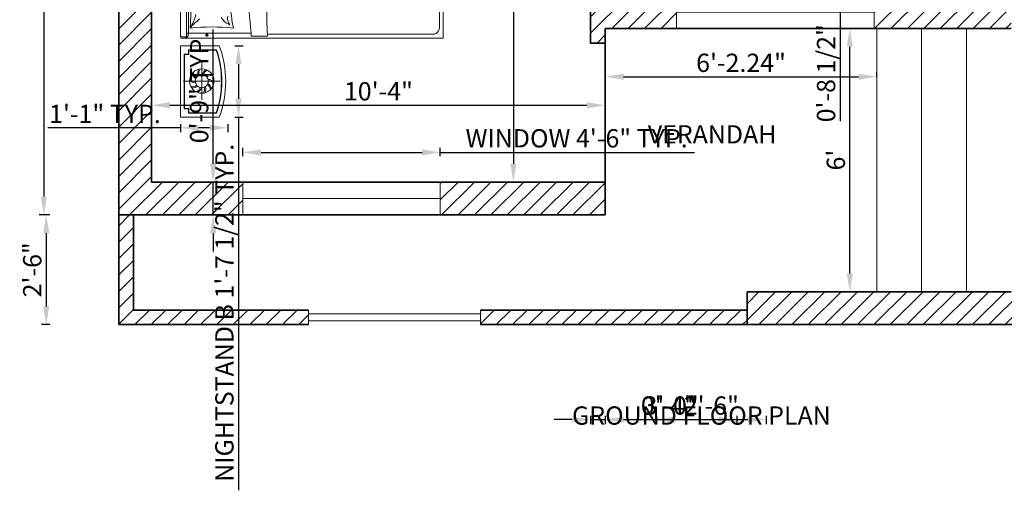
# Model space of a CAD drawing. Units: inches. Extents: x -196 to 219, y -474 to 80.
# Tile 1 of 4: x -196 to 73, y -474 to -346. Entities that reach past the tile are written whole.
import ezdxf

# ---------------------------------------------------------------- set-up
doc = ezdxf.new("R2010")
doc.units = ezdxf.units.IN
doc.header["$PDMODE"] = 35
doc.header["$PDSIZE"] = 5
for name, color, linetype, lineweight in [('A-ANNO-DIMS', 2, 'Continuous', 18), ('A-ANNO-TEXT', 7, 'Continuous', 18), ('A-AREA-IDEN', 7, 'Continuous', 25), ('A-FLOR-STRS', 3, 'Continuous', 18), ('A-GLAZ', 4, 'Continuous', 18), ('A-WALL', 7, 'Continuous', 35), ('A-WALL-PATT', 252, 'Continuous', 13), ('A-WALL-SITE', 7, 'Continuous', 35), ('furn', 28, 'Continuous', 18)]:
    doc.layers.add(name, color=color, linetype=linetype, lineweight=lineweight)
doc.styles.get("Standard").update_dxf_attribs({"font": 'arial.ttf'})
doc.dimstyles.new('ISO-25', dxfattribs={"dimtxt": 5, "dimasz": 5, "dimexe": 1.25, "dimexo": 0.625, "dimtad": 1, "dimlunit": 3, "dimtxsty": 'Standard', "dimcen": 2.5, "dimadec": 0, "dimazin": 0, "dimtfac": 1, "dimtmove": 0, "dimatfit": 3, "dimfxl": 1, "dimfxlon": 1, "dimarcsym": 0})
pattern_1 = [(45, (-560.5042, 72.7454), (-2.245064, 2.245064), [])]

# ---------------------------------------------------------------- blocks, each defined once
blk = doc.blocks.new('*D18')
at = {"layer": 'A-ANNO-DIMS', "color": 0, "lineweight": -2, "transparency": 16777216}
for p, q in [((-61.81, -252.09), (-59.56, -252.09)), ((-60.81, -257.09), (-60.81, -385.09)), ((-61.81, -390.09), (-59.56, -390.09))]:
    blk.add_line(p, q, dxfattribs=at)
at = {"layer": 'A-ANNO-DIMS', "color": 0, "transparency": 16777216}
for points in [[(-61.65, -257.09), (-59.98, -257.09), (-60.81, -252.09)], [(-61.65, -385.09), (-59.98, -385.09), (-60.81, -390.09)]]:
    blk.add_solid(points, dxfattribs=at)
at = {"layer": 'Defpoints', "color": 0, "transparency": 16777216}
for p in [(-159.7, -252.09), (-159.7, -390.09), (-60.81, -390.09)]:
    blk.add_point(p, dxfattribs=at)
at = {"layer": 'A-ANNO-DIMS', "color": 0, "transparency": 16777216, "insert": (-63.99, -321.09), "char_height": 5, "attachment_point": 5, "rotation": 90}
blk.add_mtext('11\'-6"', dxfattribs=at)
blk = doc.blocks.new('*D19')
at = {"layer": 'A-ANNO-DIMS', "color": 0, "lineweight": -2, "transparency": 16777216}
for p, q in [((-159.7, -370.09), (-159.7, -367.84)), ((-35.7, -370.09), (-35.7, -367.84)), ((-154.7, -369.09), (-40.7, -369.09))]:
    blk.add_line(p, q, dxfattribs=at)
at = {"layer": 'A-ANNO-DIMS', "color": 0, "transparency": 16777216}
for points in [[(-154.7, -368.26), (-154.7, -369.93), (-159.7, -369.09)], [(-40.7, -368.26), (-40.7, -369.93), (-35.7, -369.09)]]:
    blk.add_solid(points, dxfattribs=at)
at = {"layer": 'Defpoints', "color": 0, "transparency": 16777216}
for p in [(-35.7, -369.09), (-159.7, -390.09), (-35.7, -390.09)]:
    blk.add_point(p, dxfattribs=at)
at = {"layer": 'A-ANNO-DIMS', "color": 0, "transparency": 16777216, "insert": (-97.7, -365.92), "char_height": 5, "attachment_point": 5}
blk.add_mtext('10\'-4"', dxfattribs=at)
blk = doc.blocks.new('*D26')
at = {"layer": 'A-ANNO-DIMS', "color": 0, "lineweight": -2, "transparency": 16777216}
for p, q in [((-188.18, 32.91), (-190.43, 32.91)), ((-189.18, 27.91), (-189.18, -394.09)), ((-188.18, -399.09), (-190.43, -399.09))]:
    blk.add_line(p, q, dxfattribs=at)
at = {"layer": 'A-ANNO-DIMS', "color": 0, "transparency": 16777216}
for points in [[(-190.01, 27.91), (-188.35, 27.91), (-189.18, 32.91)], [(-190.01, -394.09), (-188.35, -394.09), (-189.18, -399.09)]]:
    blk.add_solid(points, dxfattribs=at)
at = {"layer": 'Defpoints', "color": 0, "transparency": 16777216}
for p in [(-168.7, 32.91), (-189.18, -399.09), (-168.7, -399.09)]:
    blk.add_point(p, dxfattribs=at)
at = {"layer": 'A-ANNO-DIMS', "color": 0, "transparency": 16777216, "insert": (-192.36, -183.09), "char_height": 5, "attachment_point": 5, "rotation": 90}
blk.add_mtext("36'", dxfattribs=at)
blk = doc.blocks.new('*D29')
at = {"layer": 'A-ANNO-DIMS', "color": 0, "lineweight": -2, "transparency": 16777216}
for p, q in [((32.16, -348.09), (29.91, -348.09)), ((31.16, -415.09), (31.16, -353.09)), ((32.16, -420.09), (29.91, -420.09))]:
    blk.add_line(p, q, dxfattribs=at)
at = {"layer": 'A-ANNO-DIMS', "color": 0, "transparency": 16777216}
for points in [[(30.33, -353.09), (31.99, -353.09), (31.16, -348.09)], [(30.33, -415.09), (31.99, -415.09), (31.16, -420.09)]]:
    blk.add_solid(points, dxfattribs=at)
at = {"layer": 'Defpoints', "color": 0, "transparency": 16777216}
for p in [(31.16, -348.09), (38.54, -348.09), (38.54, -420.09)]:
    blk.add_point(p, dxfattribs=at)
at = {"layer": 'A-ANNO-DIMS', "color": 0, "transparency": 16777216, "insert": (27.98, -384.09), "char_height": 5, "width": 4.6282, "attachment_point": 5, "rotation": 90}
blk.add_mtext("6'", dxfattribs=at)
blk = doc.blocks.new('*D30')
at = {"layer": 'A-ANNO-DIMS', "color": 0, "lineweight": -2, "transparency": 16777216}
for p, q in [((-35.7, -360.3), (-35.7, -362.55)), ((38.54, -361.3), (38.54, -360.05)), ((-30.7, -361.3), (33.54, -361.3))]:
    blk.add_line(p, q, dxfattribs=at)
at = {"layer": 'A-ANNO-DIMS', "color": 0, "transparency": 16777216}
for points in [[(-30.7, -360.47), (-30.7, -362.14), (-35.7, -361.3)], [(33.54, -360.47), (33.54, -362.14), (38.54, -361.3)]]:
    blk.add_solid(points, dxfattribs=at)
at = {"layer": 'Defpoints', "color": 0, "transparency": 16777216}
for p in [(-35.7, -357.68), (38.54, -361.3), (38.54, -361.3)]:
    blk.add_point(p, dxfattribs=at)
at = {"layer": 'A-ANNO-DIMS', "color": 0, "transparency": 16777216, "insert": (1.42, -358.13), "char_height": 5, "attachment_point": 5}
blk.add_mtext('6\'-2.24"', dxfattribs=at)
blk = doc.blocks.new('*D31')
at = {"layer": 'A-ANNO-DIMS', "color": 0, "lineweight": -2, "transparency": 16777216}
for p, q in [((-187.52, -399.09), (-189.77, -399.09)), ((-188.52, -404.09), (-188.52, -424.09)), ((-187.52, -429.09), (-189.77, -429.09))]:
    blk.add_line(p, q, dxfattribs=at)
at = {"layer": 'A-ANNO-DIMS', "color": 0, "transparency": 16777216}
for points in [[(-189.35, -404.09), (-187.68, -404.09), (-188.52, -399.09)], [(-189.35, -424.09), (-187.68, -424.09), (-188.52, -429.09)]]:
    blk.add_solid(points, dxfattribs=at)
at = {"layer": 'Defpoints', "color": 0, "transparency": 16777216}
for p in [(-168.7, -399.09), (-188.52, -429.09), (-168.7, -429.09)]:
    blk.add_point(p, dxfattribs=at)
at = {"layer": 'A-ANNO-DIMS', "color": 0, "transparency": 16777216, "insert": (-191.69, -414.09), "char_height": 5, "attachment_point": 5, "rotation": 90}
blk.add_mtext('2\'-6"', dxfattribs=at)
blk = doc.blocks.new('BED-DOUBLE')
for p, q in [((70.2, 59.88), (52.52, 59.88)), ((69.67, 60.18), (69.67, 1.06)), ((70.2, 1.4), (50.22, 1.4))]:
    blk.add_line(p, q)
for points in [[(71.86, 61.24), (0, 61.24), (0, 0), (71.86, 0)], [(71.86, 0.57), (70.2, 0.57), (70.2, 60.89), (71.86, 60.89), (71.86, 0)]]:
    blk.add_lwpolyline(points)
for points in [[(48.05, 60.18), (2.83, 60.18, 0.414214), (1.06, 58.41), (1.06, 2.83, 0.414214), (2.83, 1.06), (40.4, 1.06)], [(25.84, 40.29, 0.091296), (26.93, 45.48, 0.091296), (30.19, 41.3, 0.091296)], [(27.91, 41.58, 0.111006), (21.62, 31.47, 0.119549), (31.85, 25.09, 0.107813), (38.17, 35.17)], [(38.16, 35.23, 0.121865), (27.91, 41.58, 0.121865)], [(10.11, 32.11, 0.091296), (8.3, 37.09, 0.091296), (13.27, 35.26, 0.091296)], [(36.77, 37.19, 0.091296), (41.96, 36.12, 0.091296), (37.79, 32.85, 0.091296)], [(11.19, 34.3, 0.111006), (11.2, 22.39, 0.119549), (23.25, 22.39, 0.033212), (23.81, 26.05)], [(22.76, 29.38, 0.091296), (17.57, 30.45, 0.091296), (21.75, 33.72)], [(17.57, 30.45, 0.159461), (20.01, 29.08, -0.076283), (21.52, 28, 0.115075), (28.65, 23.55, -0.076283), (30.29, 22.67, 0.159461), (32.6, 21.09)], [(13.27, 21.22, 0.091296), (8.3, 19.39, 0.091296), (10.11, 24.37)], [(24.18, 24.37, 0.091296), (26, 19.39, 0.091296), (21.02, 21.22, 0.091296)], [(33.69, 26.28, 0.091296), (32.6, 21.09, 0.091296), (29.35, 25.28, 0.091296)], [(8.3, 19.39, 0.159461), (11.08, 19.51, -0.076283), (12.94, 19.39, 0.115075), (21.35, 19.39, -0.076283), (23.21, 19.51, 0.159461), (26, 19.39)]]:
    blk.add_lwpolyline(points, format="xyb")
for points in [[(52.52, 60.71), (52.52, 59.88, -0.072944), (50.05, 0.57), (40.23, 0.57, 0.092568), (48.02, 60.71)], [(57.36, 58.53, 0.058596), (69.19, 58.53, 0.036889), (69.19, 31.42, 0.052163), (57.36, 31.42, 0.093111)], [(57.36, 29.66, 0.058596), (69.19, 29.66, 0.036648), (69.19, 2.37, 0.052163), (57.36, 2.37, 0.036967)]]:
    blk.add_lwpolyline(points, format="xyb", close=True)
for centre, radius, start, end in [((70.74, 60.18), 1.06, 90, 180), ((56.26, 55.91), 2.69, 346.4823, 38.5563), ((57.08, 53.87), 3.93, 24.2916, 70.9896), ((58.12, 67.4), 14.18, 306.4935, 321.2792), ((79.08, 52.23), 11.72, 147.5379, 167.5233), ((65.82, 51.76), 2.94, 245.8927, 286.1192), ((62.17, 43.24), 6.56, 6.6849, 58.3182), ((29.97, 42.18), 4.49, 132.6522, 168.8929), ((12.27, 9.6), 38.76, 48.3818, 67.7644), ((37.6, 28.47), 18.5, 135.1307, 161.3884), ((20.09, 45.81), 6.15, 315.7718, 333.2208), ((65.9, 36.61), 4.6, 51.8174, 79.8987), ((42.31, 42.96), 6.15, 225.5854, 243.0343), ((57.86, 39.62), 0.992, 263.7543, 347.2187), ((49.13, 50.55), 14.78, 306.2085, 315.0849), ((12.62, 35.9), 4.49, 164.5791, 200.8198), ((9.5, 32.77), 4.49, 69.3666, 105.6073), ((11.62, 43.09), 6.15, 265.0387, 282.4877), ((17.27, 9.95), 25.09, 83.1956, 104.0284), ((17.15, 19.08), 18.5, 76.8711, 103.1289), ((38.65, 33.09), 4.49, 42.4658, 78.7065), ((37.79, 37.3), 4.33, 307.2937, 344.0973), ((53.97, 34.88), 4.84, 314.406, 6.8342), ((65.25, 30.79), 4.95, 40.5354, 70.3558), ((26.34, 28.3), 18.5, 167.0576, 193.3153), ((2.31, 33.75), 6.15, 347.6988, 5.1477), ((22.41, 28.73), 5.13, 128.7754, 160.3571), ((14.27, 36.4), 6.15, 323.2983, 340.7472), ((45.34, 30.19), 6.15, 143.2983, 160.7472), ((55.66, 33.97), 3.07, 303.6349, 0.8456), ((61.08, 27.7), 8.92, 24.6457, 44.1585), ((22.01, 38.11), 18.5, 315.1307, 341.3884), ((58.12, 38.53), 14.18, 306.4935, 321.2792), ((79.08, 23.37), 11.72, 147.5379, 167.5233), ((56.26, 27.04), 2.69, 346.4823, 38.5563), ((57.08, 25), 3.93, 24.2916, 70.9896), ((8.01, 28.24), 18.5, 347.0576, 348.7033), ((39.53, 20.78), 6.15, 135.7718, 153.2208), ((13.31, 20.48), 5.13, 160.7023, 192.284), ((2.34, 22.69), 6.15, 355.2252, 12.6741), ((32.04, 22.79), 6.15, 167.6988, 185.1477), ((22.07, 20.71), 4.14, 341.3996, 21.5774), ((29.96, 24.29), 4.14, 309.4726, 349.6505), ((65.82, 22.89), 2.94, 245.8927, 286.1192), ((62.17, 14.37), 6.56, 6.6849, 58.3182), ((49.13, 21.68), 14.78, 306.2085, 315.0849), ((65.9, 7.74), 4.6, 51.8174, 79.8987), ((57.86, 10.75), 0.992, 263.7543, 347.2187), ((53.97, 6.01), 4.84, 314.406, 6.8342), ((65.25, 1.92), 4.95, 40.5354, 70.3558), ((55.66, 5.1), 3.07, 303.6349, 0.8456), ((61.08, -1.17), 8.92, 24.6457, 44.1585), ((70.74, 1.06), 1.06, 180, 270)]:
    blk.add_arc(centre, radius, start, end)
blk = doc.blocks.new('NIGHTSTAND-B')
for p, q in [((6.53, 14.74), (6.53, 4.53)), ((1.42, 9.63), (11.63, 9.63))]:
    blk.add_line(p, q)
blk.add_lwpolyline([(1.77, 19.47), (12.39, 19.47), (12.39, 0), (1.77, 0, -0.181818)], format="xyb", close=True)
for points in [[(10.16, 1.06), (2.51, 1.06, -0.167087), (2.51, 18.41), (10.16, 18.41)], [(10.16, 1.17), (2.59, 1.17, -0.165559), (2.59, 18.3), (10.16, 18.3)]]:
    blk.add_lwpolyline(points, format="xyb")
for points in [[(11.33, 17.13), (10.05, 17.13), (10.05, 18.41)], [(11.33, 17.24), (10.16, 17.24), (10.16, 18.41)], [(11.22, 17.24), (11.22, 2.23)], [(11.33, 17.24), (11.33, 2.23)], [(11.33, 2.34), (10.05, 2.34), (10.05, 1.06)], [(11.33, 2.23), (10.16, 2.23), (10.16, 1.06)]]:
    blk.add_lwpolyline(points)
for radius in [3.33, 1.81]:
    blk.add_circle((6.53, 9.63), radius)
for centre, radius, start, end in [((6.04, 12.1), 2.14, 190.17, 236.4897), ((5.85, 11.99), 1.63, 178.3002, 238.538), ((7.58, 11.92), 2.14, 154.17, 200.4897), ((7.37, 11.94), 1.63, 142.3002, 202.538), ((8.72, 10.86), 2.14, 118.17, 164.4897), ((8.56, 11), 1.63, 106.3002, 166.538), ((9.03, 9.34), 2.14, 82.17, 128.4897), ((8.98, 9.55), 1.63, 70.3002, 130.538), ((4.68, 11.34), 2.14, 226.17, 272.4897), ((4.6, 11.14), 1.63, 214.3002, 274.538), ((4.08, 9.72), 1.63, 250.3002, 310.538), ((4.03, 9.93), 2.14, 262.17, 308.4897), ((5.47, 7.35), 2.14, 334.17, 20.4897), ((7.2, 7.28), 1.63, 358.3002, 58.538), ((7.02, 7.17), 2.14, 10.17, 56.4897), ((8.37, 7.93), 2.14, 46.17, 92.4897), ((8.46, 8.12), 1.63, 34.3002, 94.538), ((4.49, 8.26), 1.63, 286.3002, 346.538), ((4.33, 8.4), 2.14, 298.17, 344.4897), ((5.69, 7.33), 1.63, 322.3002, 22.538)]:
    blk.add_arc(centre, radius, start, end)
blk = doc.blocks.new('WIN-54IN')
for p, q in [((0, 9), (0, 0)), ((54, 9), (54, 0)), ((0, 4.5), (54, 4.5))]:
    blk.add_line(p, q)
blk = doc.blocks.new('*D42')
at = {"layer": 'A-ANNO-DIMS', "color": 0, "lineweight": -2, "transparency": 16777216}
for p, q in [((-136.95, -352.85), (-134.7, -352.85)), ((-135.95, -357.85), (-135.95, -367.32)), ((-136.95, -372.32), (-134.7, -372.32)), ((-135.95, -372.32), (-135.95, -474.4))]:
    blk.add_line(p, q, dxfattribs=at)
at = {"layer": 'A-ANNO-DIMS', "color": 0, "transparency": 16777216}
for points in [[(-136.78, -357.85), (-135.11, -357.85), (-135.95, -352.85)], [(-136.78, -367.32), (-135.11, -367.32), (-135.95, -372.32)]]:
    blk.add_solid(points, dxfattribs=at)
at = {"layer": 'Defpoints', "color": 0, "transparency": 16777216}
for p in [(-138.87, -352.85), (-138.87, -372.32), (-135.95, -372.32)]:
    blk.add_point(p, dxfattribs=at)
at = {"layer": 'A-ANNO-DIMS', "color": 0, "transparency": 16777216, "insert": (-139.16, -425.86), "char_height": 5, "attachment_point": 5, "rotation": 90}
blk.add_mtext('NIGHTSTAND B 1\'-7 1/2" TYP.', dxfattribs=at)
blk = doc.blocks.new('*D43')
at = {"layer": 'A-ANNO-DIMS', "color": 0, "lineweight": -2, "transparency": 16777216}
for p, q in [((-151.85, -375.24), (-188.1, -375.24)), ((-151.85, -374.24), (-151.85, -376.49)), ((-143.87, -375.24), (-146.85, -375.24)), ((-138.87, -374.24), (-138.87, -376.49))]:
    blk.add_line(p, q, dxfattribs=at)
at = {"layer": 'A-ANNO-DIMS', "color": 0, "transparency": 16777216}
for points in [[(-146.85, -374.41), (-146.85, -376.08), (-151.85, -375.24)], [(-143.87, -374.41), (-143.87, -376.08), (-138.87, -375.24)]]:
    blk.add_solid(points, dxfattribs=at)
at = {"layer": 'Defpoints', "color": 0, "transparency": 16777216}
for p in [(-151.85, -372.32), (-138.87, -372.32), (-151.85, -375.24)]:
    blk.add_point(p, dxfattribs=at)
at = {"layer": 'A-ANNO-DIMS', "color": 0, "transparency": 16777216, "insert": (-172.47, -372.11), "char_height": 5, "attachment_point": 5}
blk.add_mtext('1\'-1" TYP.', dxfattribs=at)
blk = doc.blocks.new('*D46')
at = {"layer": 'A-ANNO-DIMS', "color": 0, "lineweight": -2, "transparency": 16777216}
for p, q in [((-134.79, -382.99), (-134.79, -380.74)), ((-129.79, -381.99), (-85.79, -381.99)), ((-80.79, -382.99), (-80.79, -380.74)), ((-80.79, -381.99), (-11.26, -381.99))]:
    blk.add_line(p, q, dxfattribs=at)
at = {"layer": 'A-ANNO-DIMS', "color": 0, "transparency": 16777216}
for points in [[(-129.79, -381.16), (-129.79, -382.83), (-134.79, -381.99)], [(-85.79, -381.16), (-85.79, -382.83), (-80.79, -381.99)]]:
    blk.add_solid(points, dxfattribs=at)
at = {"layer": 'Defpoints', "color": 0, "transparency": 16777216}
for p in [(-80.79, -381.99), (-134.79, -390.09), (-80.79, -390.09)]:
    blk.add_point(p, dxfattribs=at)
at = {"layer": 'A-ANNO-DIMS', "color": 0, "transparency": 16777216, "insert": (-43.53, -378.78), "char_height": 5, "attachment_point": 5}
blk.add_mtext('WINDOW 4\'-6" TYP.', dxfattribs=at)
blk = doc.blocks.new('*D47')
at = {"layer": 'A-ANNO-DIMS', "color": 0, "lineweight": -2, "transparency": 16777216}
for p, q in [((-142.89, -385.09), (-142.89, -348.37)), ((-141.89, -390.09), (-144.14, -390.09)), ((-142.89, -399.09), (-142.89, -390.09)), ((-141.89, -399.09), (-144.14, -399.09)), ((-142.89, -404.09), (-142.89, -409.09))]:
    blk.add_line(p, q, dxfattribs=at)
at = {"layer": 'A-ANNO-DIMS', "color": 0, "transparency": 16777216}
for points in [[(-143.72, -385.09), (-142.05, -385.09), (-142.89, -390.09)], [(-143.72, -404.09), (-142.05, -404.09), (-142.89, -399.09)]]:
    blk.add_solid(points, dxfattribs=at)
at = {"layer": 'Defpoints', "color": 0, "transparency": 16777216}
for p in [(-142.89, -390.09), (-134.79, -390.09), (-134.79, -399.09)]:
    blk.add_point(p, dxfattribs=at)
at = {"layer": 'A-ANNO-DIMS', "color": 0, "transparency": 16777216, "insert": (-146.06, -364.23), "char_height": 5, "attachment_point": 5, "rotation": 90}
blk.add_mtext('0\'-9" TYP.', dxfattribs=at)
blk = doc.blocks.new('*D55')
at = {"layer": 'A-ANNO-DIMS', "color": 0, "lineweight": -2, "transparency": 16777216}
for p, q in [((28.52, -323.75), (28.52, -318.75)), ((27.52, -328.75), (29.77, -328.75)), ((28.52, -328.75), (28.52, -337.25)), ((27.52, -337.25), (29.77, -337.25)), ((28.52, -342.25), (28.52, -373.44))]:
    blk.add_line(p, q, dxfattribs=at)
at = {"layer": 'A-ANNO-DIMS', "color": 0, "transparency": 16777216}
for points in [[(27.69, -323.75), (29.36, -323.75), (28.52, -328.75)], [(27.69, -342.25), (29.36, -342.25), (28.52, -337.25)]]:
    blk.add_solid(points, dxfattribs=at)
at = {"layer": 'Defpoints', "color": 0, "transparency": 16777216}
for p in [(26.72, -328.75), (26.72, -337.25), (28.52, -337.25)]:
    blk.add_point(p, dxfattribs=at)
at = {"layer": 'A-ANNO-DIMS', "color": 0, "transparency": 16777216, "insert": (25.31, -360.34), "char_height": 5, "attachment_point": 5, "rotation": 90}
blk.add_mtext('0\'-8 1/2"', dxfattribs=at)
blk = doc.blocks.new('*D57')
at = {"layer": 'A-ANNO-DIMS', "color": 0, "lineweight": -2, "transparency": 16777216}
for p, q in [((-35.7, -454.04), (-35.7, -456.29)), ((0.3, -454.04), (0.3, -456.29)), ((-30.7, -455.04), (-4.7, -455.04))]:
    blk.add_line(p, q, dxfattribs=at)
at = {"layer": 'A-ANNO-DIMS', "color": 0, "transparency": 16777216}
for points in [[(-30.7, -454.21), (-30.7, -455.88), (-35.7, -455.04)], [(-4.7, -454.21), (-4.7, -455.88), (0.3, -455.04)]]:
    blk.add_solid(points, dxfattribs=at)
at = {"layer": 'Defpoints', "color": 0, "transparency": 16777216}
for p in [(-35.7, -243.09), (0.3, -243.09), (0.3, -455.04)]:
    blk.add_point(p, dxfattribs=at)
at = {"layer": 'A-ANNO-DIMS', "color": 0, "transparency": 16777216, "insert": (-17.7, -451.86), "char_height": 5, "attachment_point": 5}
blk.add_mtext('3\'-0"', dxfattribs=at)
blk = doc.blocks.new('*D58')
at = {"layer": 'A-ANNO-DIMS', "color": 0, "lineweight": -2, "transparency": 16777216}
for p, q in [((-21.7, -454.04), (-21.7, -456.29)), ((8.3, -454.04), (8.3, -456.29)), ((-16.7, -455.04), (3.3, -455.04))]:
    blk.add_line(p, q, dxfattribs=at)
at = {"layer": 'A-ANNO-DIMS', "color": 0, "transparency": 16777216}
for points in [[(-16.7, -454.21), (-16.7, -455.88), (-21.7, -455.04)], [(3.3, -454.21), (3.3, -455.88), (8.3, -455.04)]]:
    blk.add_solid(points, dxfattribs=at)
at = {"layer": 'Defpoints', "color": 0, "transparency": 16777216}
for p in [(-21.7, -60.09), (8.3, -64.09), (8.3, -455.04)]:
    blk.add_point(p, dxfattribs=at)
at = {"layer": 'A-ANNO-DIMS', "color": 0, "transparency": 16777216, "insert": (-6.7, -451.87), "char_height": 5, "attachment_point": 5}
blk.add_mtext('2\'-6"', dxfattribs=at)
blk = doc.blocks.new('*D60')
at = {"layer": 'A-ANNO-DIMS', "color": 0, "lineweight": -2, "transparency": 16777216}
for p, q in [((61.3, 73.61), (56.3, 73.61)), ((66.3, 72.61), (66.3, 74.86)), ((66.3, 73.61), (75.3, 73.61)), ((75.3, 72.61), (75.3, 74.86)), ((80.3, 73.61), (99.84, 73.61))]:
    blk.add_line(p, q, dxfattribs=at)
at = {"layer": 'A-ANNO-DIMS', "color": 0, "transparency": 16777216}
for points in [[(61.3, 74.45), (61.3, 72.78), (66.3, 73.61)], [(80.3, 74.45), (80.3, 72.78), (75.3, 73.61)]]:
    blk.add_solid(points, dxfattribs=at)
at = {"layer": 'Defpoints', "color": 0, "transparency": 16777216}
for p in [(75.3, 73.61), (66.3, -339.09), (75.3, -348.09)]:
    blk.add_point(p, dxfattribs=at)
at = {"layer": 'A-ANNO-DIMS', "color": 0, "transparency": 16777216, "insert": (92.57, 76.79), "char_height": 5, "attachment_point": 5}
blk.add_mtext('0\'-9"', dxfattribs=at)
blk = doc.blocks.new('*D61')
at = {"layer": 'A-ANNO-DIMS', "color": 0, "lineweight": -2, "transparency": 16777216}
for p, q in [((-39.7, -454.04), (-39.7, -456.29)), ((-35.7, -454.04), (-35.7, -456.29)), ((-44.7, -455.04), (-49.7, -455.04)), ((-39.7, -455.04), (-35.7, -455.04)), ((-30.7, -455.04), (-11.16, -455.04))]:
    blk.add_line(p, q, dxfattribs=at)
at = {"layer": 'A-ANNO-DIMS', "color": 0, "transparency": 16777216}
for points in [[(-44.7, -454.21), (-44.7, -455.88), (-39.7, -455.04)], [(-30.7, -454.21), (-30.7, -455.88), (-35.7, -455.04)]]:
    blk.add_solid(points, dxfattribs=at)
at = {"layer": 'Defpoints', "color": 0, "transparency": 16777216}
for p in [(-35.7, -243.09), (-39.7, -252.09), (-35.7, -455.04)]:
    blk.add_point(p, dxfattribs=at)
at = {"layer": 'A-ANNO-DIMS', "color": 0, "transparency": 16777216, "insert": (-18.43, -451.87), "char_height": 5, "attachment_point": 5}
blk.add_mtext('0\'-4"', dxfattribs=at)

msp = doc.modelspace()

# ---------------------------------------------------------------- hatches: boundary and pattern name
at = {"layer": 'A-WALL-PATT'}
h = msp.add_hatch(dxfattribs=at)
h.set_pattern_fill('ANSI31', color=256)
h.set_pattern_definition(pattern_1)
h.paths.add_polyline_path([(-159.698, -243.094), (-159.698, -148.094), (-159.698, 23.906), (-39.698, 23.906), (-39.698, -108.969), (-35.698, -108.969), (-35.698, -105.094), (-23.894, -105.094), (-23.894, -96.094), (-35.698, -96.094), (-35.698, -64.094), (-21.698, -64.094), (-21.698, -60.094), (-35.698, -60.094), (-35.698, -12.094), (-24.951, -12.094), (-24.951, -8.094), (-35.698, -8.094), (-35.698, 23.906), (-35.698, 27.906), (60.302, 27.906), (60.302, 23.906), (60.302, -8.094), (42.302, -8.094), (42.302, -12.094), (60.302, -12.094), (60.302, -96.094), (42.302, -96.094), (8.302, -96.094), (8.302, -105.094), (42.302, -105.094), (60.302, -105.094), (64.302, -105.094), (64.302, 23.906), (182.302, 23.906), (182.302, -96.094), (100.302, -96.094), (100.302, -105.094), (182.302, -105.094), (182.302, -252.094), (191.302, -252.094), (191.302, 32.906), (-168.698, 32.906), (-168.698, -399.094), (-134.786, -399.094), (-134.786, -390.094), (-159.698, -390.094)])
h.paths.add_polyline_path([(191.302, -252.094), (187.302, -252.094), (187.302, -420.094), (183.555, -420.094), (183.555, -429.094), (191.302, -429.094)])
h.paths.add_polyline_path([(87.555, -420.094), (75.302, -420.094), (38.543, -420.094), (3.06, -420.094), (3.06, -425.094), (3.06, -429.094), (87.555, -429.094)])
h.paths.add_polyline_path([(75.302, -252.094), (81.302, -252.094), (81.302, -243.094), (0.302, -243.094), (0.302, -252.094), (66.302, -252.094), (66.302, -339.094), (37.784, -339.094), (37.784, -348.094), (66.302, -348.094), (75.302, -348.094)], flags=17)
h.paths.add_polyline_path([(-16.216, -339.094), (-35.698, -339.094), (-35.698, -243.094), (-43.698, -243.094), (-43.698, -252.094), (-39.698, -252.094), (-39.698, -352.094), (-35.698, -352.094), (-35.698, -348.094), (-16.216, -348.094)], flags=17)
h.paths.add_polyline_path([(-79.698, -243.094), (-159.698, -243.094), (-159.698, -252.094), (-79.698, -252.094)], flags=17)
h.paths.add_polyline_path([(-35.698, -144.094), (-159.698, -144.094), (-159.698, -148.094), (-35.698, -148.094)], flags=17)
h = msp.add_hatch(dxfattribs=at)
h.set_pattern_fill('ANSI31', color=256)
h.set_pattern_definition(pattern_1)
h.paths.add_polyline_path([(3.06, -425.094), (-69.82, -425.094), (-69.82, -429.094), (3.06, -429.094)])
h.paths.add_polyline_path([(-116.772, -425.094), (-164.698, -425.094), (-164.698, -399.094), (-168.698, -399.094), (-168.698, -429.094), (-116.772, -429.094)])
h.paths.add_polyline_path([(-35.698, -390.094), (-80.786, -390.094), (-80.786, -399.094), (-35.698, -399.094)])

# ---------------------------------------------------------------- linework, layer by layer
at = {"layer": 'A-FLOR-STRS'}
for p, q in [((38.543, -348.094), (38.543, -420.094)), ((50.796, -420.094), (50.796, -348.094)), ((63.049, -420.094), (63.049, -348.094))]:
    msp.add_line(p, q, dxfattribs=at)
at = {"layer": 'A-GLAZ'}
for p, q in [((-116.772, -425.094), (-116.772, -429.094)), ((-69.82, -429.094), (-69.82, -425.094)), ((-116.772, -426.094), (-69.82, -426.094)), ((-116.772, -428.094), (-69.82, -428.094))]:
    msp.add_line(p, q, dxfattribs=at)
at = {"layer": 'A-WALL'}
for p, q in [((-168.698, -399.094), (-168.698, 32.906)), ((-159.698, -390.094), (-159.698, -243.094)), ((-39.698, -352.094), (-39.698, -252.094)), ((-35.698, -390.094), (-35.698, -348.094)), ((66.302, -348.094), (-35.698, -348.094)), ((66.302, -348.094), (75.302, -348.094)), ((-35.698, -352.094), (-39.698, -352.094)), ((-35.698, -390.094), (-159.698, -390.094)), ((-35.698, -390.094), (-35.698, -399.094)), ((-35.698, -399.094), (-168.698, -399.094))]:
    msp.add_line(p, q, dxfattribs=at)
at = {"layer": 'A-WALL-SITE'}
for p, q in [((-168.698, -399.094), (-168.698, -429.094)), ((-164.698, -399.094), (-164.698, -425.094)), ((3.06, -420.094), (38.543, -420.094)), ((3.06, -425.094), (3.06, -420.094)), ((38.543, -420.094), (75.302, -420.094)), ((-164.698, -425.094), (-116.772, -425.094)), ((-69.82, -425.094), (3.06, -425.094)), ((3.06, -425.094), (3.06, -429.094)), ((-168.698, -429.094), (-116.772, -429.094)), ((-69.82, -429.094), (3.06, -429.094)), ((3.06, -429.094), (191.302, -429.094))]:
    msp.add_line(p, q, dxfattribs=at)

# ---------------------------------------------------------------- block references
at = {"layer": 'A-GLAZ'}
for p in [(-16.216, -348.094), (-134.786, -399.094)]:
    msp.add_blockref('WIN-54IN', p, dxfattribs=at)
at = {"layer": 'furn', "rotation": 180}
for name, p in [('BED-DOUBLE', (-79.99, -289.49)), ('NIGHTSTAND-B', (-139.456, -352.855))]:
    msp.add_blockref(name, p, dxfattribs=at)

# ---------------------------------------------------------------- texts
at = {"layer": 'A-ANNO-TEXT', "insert": (-44.77, -451.453), "char_height": 5, "attachment_point": 1}
msp.add_mtext_dynamic_manual_height_columns('GROUND FLOOR PLAN', width=322.9576, gutter_width=12.5, heights=[0], dxfattribs=at)
at = {"layer": 'A-AREA-IDEN', "insert": (-24.072, -374.549), "char_height": 5, "attachment_point": 1}
msp.add_mtext_dynamic_manual_height_columns('VERANDAH', width=40.8907, gutter_width=12.5, heights=[0], dxfattribs=at)

# ---------------------------------------------------------------- dimensions: what is measured, and where the dimension line sits
at = {"layer": 'A-ANNO-DIMS'}
for base, p1, p2, override, picture, middle in [((75.302, 73.612), (66.302, -339.094), (75.302, -348.094), {"dimdec": 1, "dimlfac": 1, "dimrnd": 0, "dimzin": 1, "dimdsep": 46, "dimlunit": 4, "dimfrac": 2}, '*D60', (92.573, 76.79)), ((8.302, -455.044), (-21.698, -60.094), (8.302, -64.094), {"dimdec": 1, "dimlfac": 1, "dimrnd": 0, "dimzin": 1, "dimdsep": 46, "dimlunit": 4, "dimfrac": 2}, '*D58', (-6.698, -451.866)), ((-35.698, -455.044), (-39.698, -252.094), (-35.698, -243.094), {"dimdec": 1, "dimlfac": 1, "dimrnd": 0, "dimzin": 1, "dimdsep": 46, "dimlunit": 4, "dimfrac": 2}, '*D61', (-18.427, -451.866)), ((0.302, -455.044), (-35.698, -243.094), (0.302, -243.094), {"dimdec": 1, "dimlfac": 1, "dimrnd": 0, "dimzin": 1, "dimdsep": 46, "dimlunit": 4, "dimfrac": 2}, '*D57', (-17.698, -451.864)), ((38.543, -361.303), (-35.698, -357.679), (38.543, -361.303), {"dimclrd": 0, "dimclre": 0, "dimclrt": 0}, '*D30', (1.423, -358.125)), ((-35.698, -369.094), (-159.698, -390.094), (-35.698, -390.094), {"dimclrd": 0, "dimclre": 0, "dimclrt": 0}, '*D19', (-97.698, -365.916))]:
    dim = msp.add_linear_dim(base=base, p1=p1, p2=p2, dimstyle='ISO-25', override=override, dxfattribs=at)
    dim.commit()
    dim.dimension.update_dxf_attribs({"geometry": picture, "text_midpoint": middle})
for base, p1, p2, angle, override, picture, middle in [((-189.179, -399.094), (-168.698, 32.906), (-168.698, -399.094), 90, {"dimclrd": 0, "dimclre": 0, "dimclrt": 0}, '*D26', (-192.358, -183.094)), ((-60.815, -390.094), (-159.698, -252.094), (-159.698, -390.094), 90, {"dimclrd": 0, "dimclre": 0, "dimclrt": 0}, '*D18', (-63.993, -321.094)), ((28.524, -337.245), (26.724, -328.746), (26.724, -337.245), 270, {"dimdec": 1, "dimlfac": 1, "dimrnd": 0, "dimzin": 1, "dimdsep": 46, "dimlunit": 4, "dimfrac": 2}, '*D55', (25.313, -360.341)), ((31.161, -348.094), (38.543, -420.094), (38.543, -348.094), 90, {"dimclrd": 0, "dimclre": 0, "dimclrt": 0}, '*D29', (27.983, -384.094)), ((-188.517, -429.094), (-168.698, -399.094), (-168.698, -429.094), 90, {"dimclrd": 0, "dimclre": 0, "dimclrt": 0}, '*D31', (-191.695, -414.094))]:
    dim = msp.add_linear_dim(base=base, p1=p1, p2=p2, angle=angle, dimstyle='ISO-25', override=override, dxfattribs=at)
    dim.commit()
    dim.dimension.update_dxf_attribs({"geometry": picture, "text_midpoint": middle})
for base, p1, p2, angle, text, picture, middle in [((-142.886, -390.094), (-134.786, -399.094), (-134.786, -390.094), 90, '<> TYP.', '*D47', (-146.063, -364.23)), ((-135.946, -372.324), (-138.866, -352.855), (-138.866, -372.324), 270, 'NIGHTSTAND B <> TYP.', '*D42', (-139.156, -425.863)), ((-151.846, -375.245), (-138.866, -372.324), (-151.846, -372.324), 180, '<> TYP.', '*D43', (-172.474, -372.108))]:
    dim = msp.add_linear_dim(base=base, p1=p1, p2=p2, angle=angle, text=text, dimstyle='ISO-25', override={"dimdec": 1, "dimlfac": 1, "dimrnd": 0, "dimzin": 1, "dimdsep": 46, "dimlunit": 4, "dimfrac": 2}, dxfattribs=at)
    dim.commit()
    dim.dimension.update_dxf_attribs({"geometry": picture, "text_midpoint": middle})
dim = msp.add_linear_dim(base=(-80.786, -381.994), p1=(-134.786, -390.094), p2=(-80.786, -390.094), text='WINDOW <> TYP.', dimstyle='ISO-25', override={"dimdec": 1, "dimlfac": 1, "dimrnd": 0, "dimzin": 1, "dimdsep": 46, "dimlunit": 4, "dimfrac": 2}, dxfattribs=at)
dim.commit()
dim.dimension.update_dxf_attribs({"geometry": '*D46', "text_midpoint": (-43.525, -378.782)})

doc.saveas('drawing.dxf')
